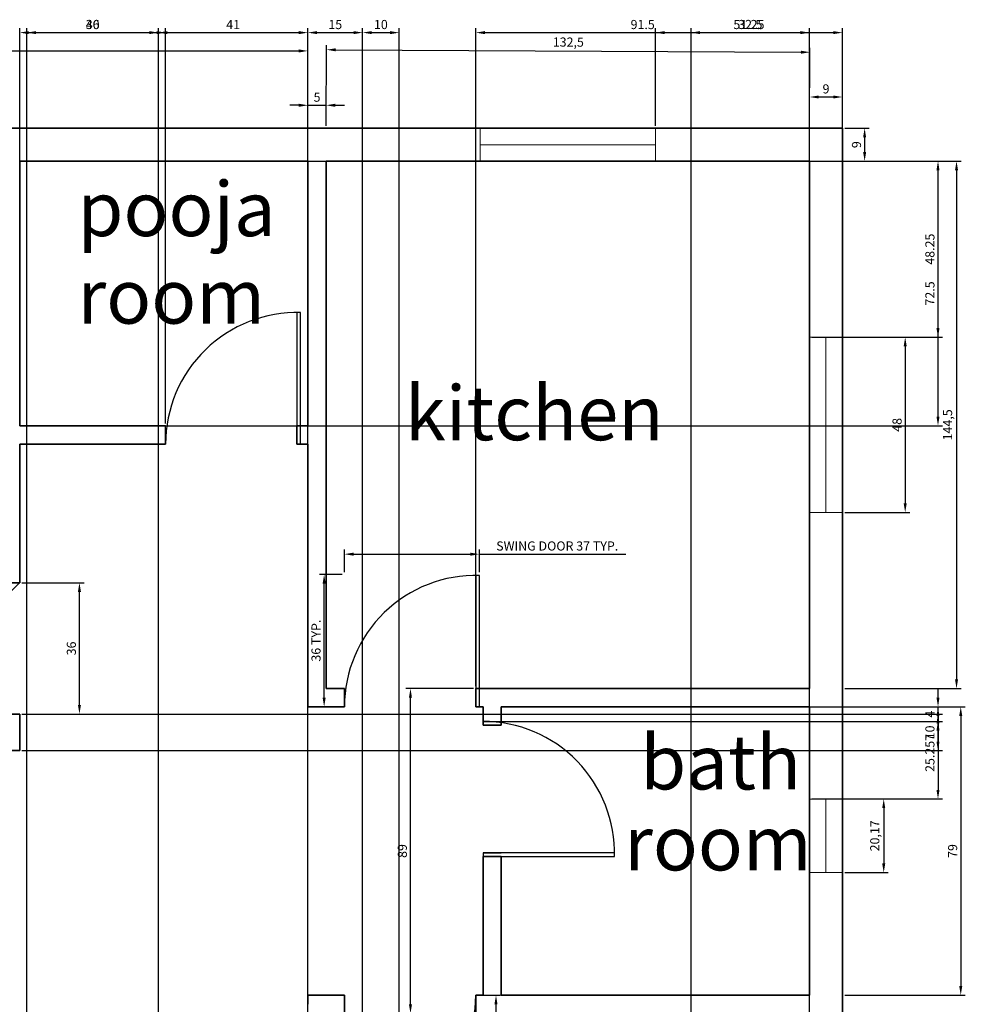
# Model space of a CAD drawing. Units: inches. Extents: x 64 to 791, y 453 to 990.
# Tile 3 of 3: x 531 to 791, y 721 to 990. Entities that reach past the tile are written whole.
import ezdxf

# ---------------------------------------------------------------- set-up
doc = ezdxf.new("R2010")
doc.units = ezdxf.units.IN
for name, color, linetype, lineweight in [('A-ANNO-DIMS', 2, 'Continuous', 18), ('A-AREA-IDEN', 7, 'Continuous', 25), ('A-DOOR', 3, 'Continuous', 25), ('A-GLAZ', 4, 'Continuous', 18), ('A-WALL', 7, 'Continuous', 35)]:
    doc.layers.add(name, color=color, linetype=linetype, lineweight=lineweight)
doc.styles.get("Standard").update_dxf_attribs({"font": 'arial.ttf'})
doc.dimstyles.new('ISO-25', dxfattribs={"dimtxt": 2.5, "dimasz": 2.5, "dimexe": 1.25, "dimexo": 0.625, "dimtad": 1, "dimtxsty": 'Standard', "dimcen": 2.5, "dimadec": 0, "dimazin": 0, "dimtfac": 1, "dimtmove": 0, "dimatfit": 3, "dimfxl": 1, "dimarcsym": 0})

# ---------------------------------------------------------------- blocks, each defined once
blk = doc.blocks.new('*D1')
at = {"layer": 'A-ANNO-DIMS', "color": 0, "lineweight": -2, "transparency": 16777216}
for p, q in [((757.56, 903.43), (775.4, 903.43)), ((774.15, 900.93), (774.15, 857.93)), ((757.56, 855.43), (775.4, 855.43))]:
    blk.add_line(p, q, dxfattribs=at)
at = {"layer": 'A-ANNO-DIMS', "color": 0, "transparency": 16777216}
for points in [[(773.73, 900.93), (774.56, 900.93), (774.15, 903.43)], [(773.73, 857.93), (774.56, 857.93), (774.15, 855.43)]]:
    blk.add_solid(points, dxfattribs=at)
at = {"layer": 'Defpoints', "color": 0, "transparency": 16777216}
for p in [(756.94, 903.43), (756.94, 855.43), (774.15, 855.43)]:
    blk.add_point(p, dxfattribs=at)
at = {"layer": 'A-ANNO-DIMS', "color": 0, "transparency": 16777216, "insert": (772.24, 879.43), "char_height": 2.5, "attachment_point": 5, "rotation": 90}
blk.add_mtext('48', dxfattribs=at)
blk = doc.blocks.new('*D2')
at = {"layer": 'A-ANNO-DIMS', "color": 0, "lineweight": -2, "transparency": 16777216}
for p, q in [((757.56, 951.68), (789.46, 951.68)), ((788.21, 949.18), (788.21, 809.68)), ((757.56, 807.18), (789.46, 807.18))]:
    blk.add_line(p, q, dxfattribs=at)
at = {"layer": 'A-ANNO-DIMS', "color": 0, "transparency": 16777216}
for points in [[(787.8, 949.18), (788.63, 949.18), (788.21, 951.68)], [(787.8, 809.68), (788.63, 809.68), (788.21, 807.18)]]:
    blk.add_solid(points, dxfattribs=at)
at = {"layer": 'Defpoints', "color": 0, "transparency": 16777216}
for p in [(756.94, 951.68), (756.94, 807.18), (788.21, 807.18)]:
    blk.add_point(p, dxfattribs=at)
at = {"layer": 'A-ANNO-DIMS', "color": 0, "transparency": 16777216, "insert": (786.09, 879.43), "char_height": 2.5, "attachment_point": 5, "rotation": 90}
blk.add_mtext('144,5', dxfattribs=at)
blk = doc.blocks.new('*D3')
at = {"layer": 'A-ANNO-DIMS', "color": 0, "lineweight": -2, "transparency": 16777216}
for p, q in [((757.56, 960.68), (764.28, 960.68)), ((763.03, 958.18), (763.03, 954.18)), ((757.56, 951.68), (764.28, 951.68))]:
    blk.add_line(p, q, dxfattribs=at)
at = {"layer": 'A-ANNO-DIMS', "color": 0, "transparency": 16777216}
for points in [[(762.61, 958.18), (763.44, 958.18), (763.03, 960.68)], [(762.61, 954.18), (763.44, 954.18), (763.03, 951.68)]]:
    blk.add_solid(points, dxfattribs=at)
at = {"layer": 'Defpoints', "color": 0, "transparency": 16777216}
for p in [(756.94, 960.68), (756.94, 951.68), (763.03, 951.68)]:
    blk.add_point(p, dxfattribs=at)
at = {"layer": 'A-ANNO-DIMS', "color": 0, "transparency": 16777216, "insert": (761.12, 956.18), "char_height": 2.5, "attachment_point": 5, "rotation": 90}
blk.add_mtext('9', dxfattribs=at)
blk = doc.blocks.new('*D4')
at = {"layer": 'A-ANNO-DIMS', "color": 0, "lineweight": -2, "transparency": 16777216}
for p, q in [((747.94, 960.63), (747.94, 970.5)), ((750.44, 969.25), (754.44, 969.25)), ((756.94, 960.63), (756.94, 970.5))]:
    blk.add_line(p, q, dxfattribs=at)
at = {"layer": 'A-ANNO-DIMS', "color": 0, "transparency": 16777216}
for points in [[(750.44, 969.66), (750.44, 968.83), (747.94, 969.25)], [(754.44, 969.66), (754.44, 968.83), (756.94, 969.25)]]:
    blk.add_solid(points, dxfattribs=at)
at = {"layer": 'Defpoints', "color": 0, "transparency": 16777216}
for p in [(756.94, 969.25), (747.94, 960), (756.94, 960)]:
    blk.add_point(p, dxfattribs=at)
at = {"layer": 'A-ANNO-DIMS', "color": 0, "transparency": 16777216, "insert": (752.44, 971.15), "char_height": 2.5, "attachment_point": 5}
blk.add_mtext('9', dxfattribs=at)
blk = doc.blocks.new('*D5')
at = {"layer": 'A-ANNO-DIMS', "color": 0, "lineweight": -2, "transparency": 16777216}
for p, q in [((615.44, 961.31), (615.55, 983.44)), ((618.05, 982.18), (745.55, 981.52)), ((747.94, 960.63), (748.05, 982.76))]:
    blk.add_line(p, q, dxfattribs=at)
at = {"layer": 'A-ANNO-DIMS', "color": 0, "transparency": 16777216}
for points in [[(618.05, 982.59), (618.05, 981.76), (615.55, 982.19)], [(745.55, 981.94), (745.55, 981.1), (748.05, 981.51)]]:
    blk.add_solid(points, dxfattribs=at)
at = {"layer": 'Defpoints', "color": 0, "transparency": 16777216}
for p in [(748.05, 981.51), (615.44, 960.68), (747.94, 960)]:
    blk.add_point(p, dxfattribs=at)
at = {"layer": 'A-ANNO-DIMS', "color": 0, "transparency": 16777216, "insert": (681.81, 983.97), "char_height": 2.5, "attachment_point": 5, "rotation": 359.7046}
blk.add_mtext('132,5', dxfattribs=at)
blk = doc.blocks.new('*D6')
at = {"layer": 'A-ANNO-DIMS', "color": 0, "lineweight": -2, "transparency": 16777216}
for p, q in [((607.94, 966.98), (605.44, 966.98)), ((610.44, 961.31), (610.44, 968.23)), ((610.44, 966.98), (615.44, 966.98)), ((615.44, 961.31), (615.44, 968.23)), ((617.94, 966.98), (620.44, 966.98))]:
    blk.add_line(p, q, dxfattribs=at)
at = {"layer": 'A-ANNO-DIMS', "color": 0, "transparency": 16777216}
for points in [[(607.94, 967.4), (607.94, 966.56), (610.44, 966.98)], [(617.94, 967.4), (617.94, 966.56), (615.44, 966.98)]]:
    blk.add_solid(points, dxfattribs=at)
at = {"layer": 'Defpoints', "color": 0, "transparency": 16777216}
for p in [(615.44, 966.98), (610.44, 960.68), (615.44, 960.68)]:
    blk.add_point(p, dxfattribs=at)
at = {"layer": 'A-ANNO-DIMS', "color": 0, "transparency": 16777216, "insert": (612.94, 968.88), "char_height": 2.5, "attachment_point": 5}
blk.add_mtext('5', dxfattribs=at)
blk = doc.blocks.new('*D7')
at = {"layer": 'A-ANNO-DIMS', "color": 0, "lineweight": -2, "transparency": 16777216}
for p, q in [((405.94, 961.31), (405.94, 983.12)), ((408.44, 981.87), (607.94, 981.87)), ((610.44, 961.31), (610.44, 983.12))]:
    blk.add_line(p, q, dxfattribs=at)
at = {"layer": 'A-ANNO-DIMS', "color": 0, "transparency": 16777216}
for points in [[(408.44, 982.28), (408.44, 981.45), (405.94, 981.87)], [(607.94, 982.28), (607.94, 981.45), (610.44, 981.87)]]:
    blk.add_solid(points, dxfattribs=at)
at = {"layer": 'Defpoints', "color": 0, "transparency": 16777216}
for p in [(610.44, 981.87), (405.94, 960.68), (610.44, 960.68)]:
    blk.add_point(p, dxfattribs=at)
at = {"layer": 'A-ANNO-DIMS', "color": 0, "transparency": 16777216, "insert": (508.19, 984), "char_height": 2.5, "attachment_point": 5}
blk.add_mtext('204,5', dxfattribs=at)
blk = doc.blocks.new('*D11')
at = {"layer": 'A-ANNO-DIMS', "color": 0, "lineweight": -2, "transparency": 16777216}
for p, q in [((757.56, 802.18), (790.62, 802.18)), ((789.37, 799.68), (789.37, 725.68)), ((757.56, 723.18), (790.62, 723.18))]:
    blk.add_line(p, q, dxfattribs=at)
at = {"layer": 'A-ANNO-DIMS', "color": 0, "transparency": 16777216}
for points in [[(788.96, 799.68), (789.79, 799.68), (789.37, 802.18)], [(788.96, 725.68), (789.79, 725.68), (789.37, 723.18)]]:
    blk.add_solid(points, dxfattribs=at)
at = {"layer": 'Defpoints', "color": 0, "transparency": 16777216}
for p in [(756.94, 802.18), (756.94, 723.18), (789.37, 723.18)]:
    blk.add_point(p, dxfattribs=at)
at = {"layer": 'A-ANNO-DIMS', "color": 0, "transparency": 16777216, "insert": (787.47, 762.68), "char_height": 2.5, "attachment_point": 5, "rotation": 90}
blk.add_mtext('79', dxfattribs=at)
blk = doc.blocks.new('*D12')
at = {"layer": 'A-ANNO-DIMS', "color": 0, "lineweight": -2, "transparency": 16777216}
for p, q in [((757.56, 776.93), (769.51, 776.93)), ((768.26, 774.43), (768.26, 759.26)), ((757.56, 756.76), (769.51, 756.76))]:
    blk.add_line(p, q, dxfattribs=at)
at = {"layer": 'A-ANNO-DIMS', "color": 0, "transparency": 16777216}
for points in [[(767.84, 774.43), (768.68, 774.43), (768.26, 776.93)], [(767.84, 759.26), (768.68, 759.26), (768.26, 756.76)]]:
    blk.add_solid(points, dxfattribs=at)
at = {"layer": 'Defpoints', "color": 0, "transparency": 16777216}
for p in [(756.94, 776.93), (756.94, 756.76), (768.26, 756.76)]:
    blk.add_point(p, dxfattribs=at)
at = {"layer": 'A-ANNO-DIMS', "color": 0, "transparency": 16777216, "insert": (766.13, 766.84), "char_height": 2.5, "attachment_point": 5, "rotation": 90}
blk.add_mtext('20,17', dxfattribs=at)
blk = doc.blocks.new('*D13')
at = {"layer": 'A-ANNO-DIMS', "color": 0, "lineweight": -2, "transparency": 16777216}
for p, q in [((532.06, 836.18), (549.07, 836.18)), ((547.82, 802.68), (547.82, 833.68)), ((532.06, 800.18), (549.07, 800.18))]:
    blk.add_line(p, q, dxfattribs=at)
at = {"layer": 'A-ANNO-DIMS', "color": 0, "transparency": 16777216}
for points in [[(547.4, 833.68), (548.23, 833.68), (547.82, 836.18)], [(547.4, 802.68), (548.23, 802.68), (547.82, 800.18)]]:
    blk.add_solid(points, dxfattribs=at)
at = {"layer": 'Defpoints', "color": 0, "transparency": 16777216}
for p in [(531.44, 836.18), (547.82, 836.18), (531.44, 800.18)]:
    blk.add_point(p, dxfattribs=at)
at = {"layer": 'A-ANNO-DIMS', "color": 0, "transparency": 16777216, "insert": (545.92, 818.18), "char_height": 2.5, "attachment_point": 5, "rotation": 90}
blk.add_mtext('36', dxfattribs=at)
blk = doc.blocks.new('*D23')
at = {"layer": 'A-ANNO-DIMS', "color": 0, "lineweight": -2, "transparency": 16777216}
for p, q in [((655.81, 807.18), (637.3, 807.18)), ((638.55, 720.68), (638.55, 804.68)), ((655.81, 718.18), (637.3, 718.18))]:
    blk.add_line(p, q, dxfattribs=at)
at = {"layer": 'A-ANNO-DIMS', "color": 0, "transparency": 16777216}
for points in [[(638.13, 804.68), (638.96, 804.68), (638.55, 807.18)], [(638.13, 720.68), (638.96, 720.68), (638.55, 718.18)]]:
    blk.add_solid(points, dxfattribs=at)
at = {"layer": 'Defpoints', "color": 0, "transparency": 16777216}
for p in [(638.55, 807.18), (656.44, 807.18), (656.44, 718.18)]:
    blk.add_point(p, dxfattribs=at)
at = {"layer": 'A-ANNO-DIMS', "color": 0, "transparency": 16777216, "insert": (636.64, 762.68), "char_height": 2.5, "attachment_point": 5, "rotation": 90}
blk.add_mtext('89', dxfattribs=at)
blk = doc.blocks.new('WIN-48IN')
for p, q in [((0, 48), (9, 48)), ((4.5, 48), (4.5, 0)), ((0, 0), (9, 0))]:
    blk.add_line(p, q)
blk = doc.blocks.new('DOOR-SWING-36IN')
for p, q in [((0, 0), (0, 5)), ((36, 0), (36, 5))]:
    blk.add_line(p, q)
blk.add_lwpolyline([(36, 0), (37, 0), (37, 36), (36, 36)], close=True)
blk.add_arc((36.01, 0), 36.01, 88.4304, 180)
blk = doc.blocks.new('DOOR-SWING-36IN-OPEN-PROFILE')
for p, q in [((0, 0), (0, 5)), ((36, 0), (36, 5))]:
    blk.add_line(p, q)
blk.add_lwpolyline([(37, 5), (37, 36), (36, 36), (36, 0), (37, 0)])
blk.add_arc((36.01, 0), 36.01, 88.4304, 180)
blk = doc.blocks.new('*D28')
at = {"layer": 'A-ANNO-DIMS', "color": 0, "lineweight": -2, "transparency": 16777216}
for p, q in [((620.44, 839.07), (620.44, 845.25)), ((657.44, 839.07), (657.44, 845.25)), ((622.94, 844), (654.94, 844)), ((657.44, 844), (697.6, 844))]:
    blk.add_line(p, q, dxfattribs=at)
at = {"layer": 'A-ANNO-DIMS', "color": 0, "transparency": 16777216}
for points in [[(622.94, 844.42), (622.94, 843.58), (620.44, 844)], [(654.94, 844.42), (654.94, 843.58), (657.44, 844)]]:
    blk.add_solid(points, dxfattribs=at)
at = {"layer": 'Defpoints', "color": 0, "transparency": 16777216}
for p in [(657.44, 844), (620.44, 838.45), (657.44, 838.45)]:
    blk.add_point(p, dxfattribs=at)
at = {"layer": 'A-ANNO-DIMS', "color": 0, "transparency": 16777216, "insert": (678.77, 845.92), "char_height": 2.5, "attachment_point": 5}
blk.add_mtext('SWING DOOR 37 TYP.', dxfattribs=at)
blk = doc.blocks.new('*D29')
at = {"layer": 'A-ANNO-DIMS', "color": 0, "lineweight": -2, "transparency": 16777216}
for p, q in [((619.81, 838.45), (613.64, 838.45)), ((614.89, 804.68), (614.89, 835.95)), ((619.81, 802.18), (613.64, 802.18))]:
    blk.add_line(p, q, dxfattribs=at)
at = {"layer": 'A-ANNO-DIMS', "color": 0, "transparency": 16777216}
for points in [[(614.47, 835.95), (615.3, 835.95), (614.89, 838.45)], [(614.47, 804.68), (615.3, 804.68), (614.89, 802.18)]]:
    blk.add_solid(points, dxfattribs=at)
at = {"layer": 'Defpoints', "color": 0, "transparency": 16777216}
for p in [(614.89, 838.45), (620.44, 838.45), (620.44, 802.18)]:
    blk.add_point(p, dxfattribs=at)
at = {"layer": 'A-ANNO-DIMS', "color": 0, "transparency": 16777216, "insert": (612.98, 820.32), "char_height": 2.5, "attachment_point": 5, "rotation": 90}
blk.add_mtext('36 TYP.', dxfattribs=at)
blk = doc.blocks.new('*D31')
at = {"layer": 'A-ANNO-DIMS', "color": 0, "lineweight": -2, "transparency": 16777216}
for p, q in [((657.06, 723.18), (663.24, 723.18)), ((661.99, 720.68), (661.99, 689.42)), ((657.06, 686.92), (663.24, 686.92))]:
    blk.add_line(p, q, dxfattribs=at)
at = {"layer": 'A-ANNO-DIMS', "color": 0, "transparency": 16777216}
for points in [[(661.57, 720.68), (662.4, 720.68), (661.99, 723.18)], [(661.57, 689.42), (662.4, 689.42), (661.99, 686.92)]]:
    blk.add_solid(points, dxfattribs=at)
at = {"layer": 'Defpoints', "color": 0, "transparency": 16777216}
for p in [(656.44, 723.18), (656.44, 686.92), (661.99, 686.92)]:
    blk.add_point(p, dxfattribs=at)
at = {"layer": 'A-ANNO-DIMS', "color": 0, "transparency": 16777216, "insert": (660.08, 705.05), "char_height": 2.5, "attachment_point": 5, "rotation": 90}
blk.add_mtext('36 TYP.', dxfattribs=at)
blk = doc.blocks.new('*D35')
at = {"layer": 'A-ANNO-DIMS', "color": 0, "lineweight": -2, "transparency": 16777216}
for p, q in [((532.06, 951.68), (784.39, 951.68)), ((783.14, 881.68), (783.14, 949.18)), ((532.06, 879.18), (784.39, 879.18))]:
    blk.add_line(p, q, dxfattribs=at)
at = {"layer": 'A-ANNO-DIMS', "color": 0, "transparency": 16777216}
for points in [[(782.72, 949.18), (783.55, 949.18), (783.14, 951.68)], [(782.72, 881.68), (783.55, 881.68), (783.14, 879.18)]]:
    blk.add_solid(points, dxfattribs=at)
at = {"layer": 'Defpoints', "color": 0, "transparency": 16777216}
for p in [(531.44, 951.68), (783.14, 951.68), (531.44, 879.18)]:
    blk.add_point(p, dxfattribs=at)
at = {"layer": 'A-ANNO-DIMS', "color": 0, "transparency": 16777216, "insert": (781.24, 915.43), "char_height": 2.5, "attachment_point": 5, "rotation": 90}
blk.add_mtext('72.5', dxfattribs=at)
blk = doc.blocks.new('*D38')
at = {"layer": 'A-ANNO-DIMS', "color": 0, "lineweight": -2, "transparency": 16777216}
for p, q in [((705.69, 961.31), (705.69, 988.13)), ((756.94, 961.31), (756.94, 988.13)), ((708.19, 986.88), (754.44, 986.88))]:
    blk.add_line(p, q, dxfattribs=at)
at = {"layer": 'A-ANNO-DIMS', "color": 0, "transparency": 16777216}
for points in [[(708.19, 987.3), (708.19, 986.47), (705.69, 986.88)], [(754.44, 987.3), (754.44, 986.47), (756.94, 986.88)]]:
    blk.add_solid(points, dxfattribs=at)
at = {"layer": 'Defpoints', "color": 0, "transparency": 16777216}
for p in [(756.94, 986.88), (705.69, 960.68), (756.94, 960.68)]:
    blk.add_point(p, dxfattribs=at)
at = {"layer": 'A-ANNO-DIMS', "color": 0, "transparency": 16777216, "insert": (731.31, 988.78), "char_height": 2.5, "attachment_point": 5}
blk.add_mtext('51.25', dxfattribs=at)
blk = doc.blocks.new('*D41')
at = {"layer": 'A-ANNO-DIMS', "color": 0, "lineweight": -2, "transparency": 16777216}
for p, q in [((748.56, 802.18), (784.39, 802.18)), ((783.14, 799.68), (783.14, 779.43)), ((748.56, 776.93), (784.39, 776.93))]:
    blk.add_line(p, q, dxfattribs=at)
at = {"layer": 'A-ANNO-DIMS', "color": 0, "transparency": 16777216}
for points in [[(782.72, 799.68), (783.55, 799.68), (783.14, 802.18)], [(782.72, 779.43), (783.55, 779.43), (783.14, 776.93)]]:
    blk.add_solid(points, dxfattribs=at)
at = {"layer": 'Defpoints', "color": 0, "transparency": 16777216}
for p in [(747.94, 802.18), (747.94, 776.93), (783.14, 776.93)]:
    blk.add_point(p, dxfattribs=at)
at = {"layer": 'A-ANNO-DIMS', "color": 0, "transparency": 16777216, "insert": (781.24, 789.55), "char_height": 2.5, "attachment_point": 5, "rotation": 90}
blk.add_mtext('25.257', dxfattribs=at)
blk = doc.blocks.new('*D42')
at = {"layer": 'A-ANNO-DIMS', "color": 0, "lineweight": -2, "transparency": 16777216}
for p, q in [((748.56, 951.68), (784.39, 951.68)), ((783.14, 905.93), (783.14, 949.18)), ((748.56, 903.43), (784.39, 903.43))]:
    blk.add_line(p, q, dxfattribs=at)
at = {"layer": 'A-ANNO-DIMS', "color": 0, "transparency": 16777216}
for points in [[(782.72, 949.18), (783.55, 949.18), (783.14, 951.68)], [(782.72, 905.93), (783.55, 905.93), (783.14, 903.43)]]:
    blk.add_solid(points, dxfattribs=at)
at = {"layer": 'Defpoints', "color": 0, "transparency": 16777216}
for p in [(747.94, 951.68), (783.14, 951.68), (747.94, 903.43)]:
    blk.add_point(p, dxfattribs=at)
at = {"layer": 'A-ANNO-DIMS', "color": 0, "transparency": 16777216, "insert": (781.24, 927.56), "char_height": 2.5, "attachment_point": 5, "rotation": 90}
blk.add_mtext('48.25', dxfattribs=at)
blk = doc.blocks.new('*D43')
at = {"layer": 'A-ANNO-DIMS', "color": 0, "lineweight": -2, "transparency": 16777216}
for p, q in [((569.44, 562.81), (569.44, 988.13)), ((610.44, 567.81), (610.44, 988.13)), ((571.94, 986.88), (607.94, 986.88))]:
    blk.add_line(p, q, dxfattribs=at)
at = {"layer": 'A-ANNO-DIMS', "color": 0, "transparency": 16777216}
for points in [[(571.94, 987.3), (571.94, 986.47), (569.44, 986.88)], [(607.94, 987.3), (607.94, 986.47), (610.44, 986.88)]]:
    blk.add_solid(points, dxfattribs=at)
at = {"layer": 'Defpoints', "color": 0, "transparency": 16777216}
for p in [(610.44, 986.88), (610.44, 567.18), (569.44, 562.18)]:
    blk.add_point(p, dxfattribs=at)
at = {"layer": 'A-ANNO-DIMS', "color": 0, "transparency": 16777216, "insert": (589.94, 988.76), "char_height": 2.5, "attachment_point": 5}
blk.add_mtext('41', dxfattribs=at)
blk = doc.blocks.new('*D44')
at = {"layer": 'A-ANNO-DIMS', "color": 0, "lineweight": -2, "transparency": 16777216}
for p, q in [((533.44, 567.81), (533.44, 988.13)), ((569.44, 562.81), (569.44, 988.13)), ((535.94, 986.88), (566.94, 986.88))]:
    blk.add_line(p, q, dxfattribs=at)
at = {"layer": 'A-ANNO-DIMS', "color": 0, "transparency": 16777216}
for points in [[(535.94, 987.3), (535.94, 986.47), (533.44, 986.88)], [(566.94, 987.3), (566.94, 986.47), (569.44, 986.88)]]:
    blk.add_solid(points, dxfattribs=at)
at = {"layer": 'Defpoints', "color": 0, "transparency": 16777216}
for p in [(569.44, 986.88), (533.44, 567.18), (569.44, 562.18)]:
    blk.add_point(p, dxfattribs=at)
at = {"layer": 'A-ANNO-DIMS', "color": 0, "transparency": 16777216, "insert": (551.44, 988.79), "char_height": 2.5, "attachment_point": 5}
blk.add_mtext('36', dxfattribs=at)
blk = doc.blocks.new('*D45')
at = {"layer": 'A-ANNO-DIMS', "color": 0, "lineweight": -2, "transparency": 16777216}
for p, q in [((625.44, 490.31), (625.44, 988.13)), ((635.44, 490.31), (635.44, 988.13)), ((627.94, 986.88), (632.94, 986.88))]:
    blk.add_line(p, q, dxfattribs=at)
at = {"layer": 'A-ANNO-DIMS', "color": 0, "transparency": 16777216}
for points in [[(627.94, 987.3), (627.94, 986.47), (625.44, 986.88)], [(632.94, 987.3), (632.94, 986.47), (635.44, 986.88)]]:
    blk.add_solid(points, dxfattribs=at)
at = {"layer": 'Defpoints', "color": 0, "transparency": 16777216}
for p in [(635.44, 986.88), (625.44, 489.68), (635.44, 489.68)]:
    blk.add_point(p, dxfattribs=at)
at = {"layer": 'A-ANNO-DIMS', "color": 0, "transparency": 16777216, "insert": (630.44, 988.78), "char_height": 2.5, "attachment_point": 5}
blk.add_mtext('10', dxfattribs=at)
blk = doc.blocks.new('*D46')
at = {"layer": 'A-ANNO-DIMS', "color": 0, "lineweight": -2, "transparency": 16777216}
for p, q in [((610.44, 490.31), (610.44, 988.13)), ((625.44, 490.31), (625.44, 988.13)), ((612.94, 986.88), (622.94, 986.88))]:
    blk.add_line(p, q, dxfattribs=at)
at = {"layer": 'A-ANNO-DIMS', "color": 0, "transparency": 16777216}
for points in [[(612.94, 987.3), (612.94, 986.47), (610.44, 986.88)], [(622.94, 987.3), (622.94, 986.47), (625.44, 986.88)]]:
    blk.add_solid(points, dxfattribs=at)
at = {"layer": 'Defpoints', "color": 0, "transparency": 16777216}
for p in [(625.44, 986.88), (610.44, 489.68), (625.44, 489.68)]:
    blk.add_point(p, dxfattribs=at)
at = {"layer": 'A-ANNO-DIMS', "color": 0, "transparency": 16777216, "insert": (617.94, 988.78), "char_height": 2.5, "attachment_point": 5}
blk.add_mtext('15', dxfattribs=at)
blk = doc.blocks.new('*D47')
at = {"layer": 'A-ANNO-DIMS', "color": 0, "lineweight": -2, "transparency": 16777216}
for p, q in [((715.44, 490.31), (715.44, 988.13)), ((747.94, 490.31), (747.94, 988.13)), ((717.94, 986.88), (745.44, 986.88))]:
    blk.add_line(p, q, dxfattribs=at)
at = {"layer": 'A-ANNO-DIMS', "color": 0, "transparency": 16777216}
for points in [[(717.94, 987.3), (717.94, 986.47), (715.44, 986.88)], [(745.44, 987.3), (745.44, 986.47), (747.94, 986.88)]]:
    blk.add_solid(points, dxfattribs=at)
at = {"layer": 'Defpoints', "color": 0, "transparency": 16777216}
for p in [(747.94, 986.88), (715.44, 489.68), (747.94, 489.68)]:
    blk.add_point(p, dxfattribs=at)
at = {"layer": 'A-ANNO-DIMS', "color": 0, "transparency": 16777216, "insert": (731.69, 988.79), "char_height": 2.5, "attachment_point": 5}
blk.add_mtext('32.5', dxfattribs=at)
blk = doc.blocks.new('*D49')
at = {"layer": 'A-ANNO-DIMS', "color": 0, "lineweight": -2, "transparency": 16777216}
for p, q in [((531.44, 879.81), (531.44, 988.13)), ((571.44, 879.81), (571.44, 988.13)), ((533.94, 986.88), (568.94, 986.88))]:
    blk.add_line(p, q, dxfattribs=at)
at = {"layer": 'A-ANNO-DIMS', "color": 0, "transparency": 16777216}
for points in [[(533.94, 987.3), (533.94, 986.47), (531.44, 986.88)], [(568.94, 987.3), (568.94, 986.47), (571.44, 986.88)]]:
    blk.add_solid(points, dxfattribs=at)
at = {"layer": 'Defpoints', "color": 0, "transparency": 16777216}
for p in [(571.44, 986.88), (531.44, 879.18), (571.44, 879.18)]:
    blk.add_point(p, dxfattribs=at)
at = {"layer": 'A-ANNO-DIMS', "color": 0, "transparency": 16777216, "insert": (551.44, 988.78), "char_height": 2.5, "attachment_point": 5}
blk.add_mtext('40', dxfattribs=at)
blk = doc.blocks.new('*D50')
at = {"layer": 'A-ANNO-DIMS', "color": 0, "lineweight": -2, "transparency": 16777216}
for p, q in [((656.44, 807.81), (656.44, 988.13)), ((747.94, 807.81), (747.94, 988.13)), ((658.94, 986.88), (745.44, 986.88))]:
    blk.add_line(p, q, dxfattribs=at)
at = {"layer": 'A-ANNO-DIMS', "color": 0, "transparency": 16777216}
for points in [[(658.94, 987.3), (658.94, 986.47), (656.44, 986.88)], [(745.44, 987.3), (745.44, 986.47), (747.94, 986.88)]]:
    blk.add_solid(points, dxfattribs=at)
at = {"layer": 'Defpoints', "color": 0, "transparency": 16777216}
for p in [(747.94, 986.88), (656.44, 807.18), (747.94, 807.18)]:
    blk.add_point(p, dxfattribs=at)
at = {"layer": 'A-ANNO-DIMS', "color": 0, "transparency": 16777216, "insert": (702.19, 988.78), "char_height": 2.5, "attachment_point": 5}
blk.add_mtext('91.5', dxfattribs=at)
blk = doc.blocks.new('*D51')
at = {"layer": 'A-ANNO-DIMS', "color": 0, "lineweight": -2, "transparency": 16777216}
for p, q in [((783.14, 804.68), (783.14, 807.18)), ((664.06, 802.18), (784.39, 802.18)), ((783.14, 798.18), (783.14, 802.18)), ((659.06, 798.18), (784.39, 798.18)), ((783.14, 795.68), (783.14, 793.18))]:
    blk.add_line(p, q, dxfattribs=at)
at = {"layer": 'A-ANNO-DIMS', "color": 0, "transparency": 16777216}
for points in [[(782.72, 804.68), (783.55, 804.68), (783.14, 802.18)], [(782.72, 795.68), (783.55, 795.68), (783.14, 798.18)]]:
    blk.add_solid(points, dxfattribs=at)
at = {"layer": 'Defpoints', "color": 0, "transparency": 16777216}
for p in [(663.44, 802.18), (783.14, 802.18), (658.44, 798.18)]:
    blk.add_point(p, dxfattribs=at)
at = {"layer": 'A-ANNO-DIMS', "color": 0, "transparency": 16777216, "insert": (781.26, 800.18), "char_height": 2.5, "attachment_point": 5, "rotation": 90}
blk.add_mtext('4', dxfattribs=at)
blk = doc.blocks.new('*D52')
at = {"layer": 'A-ANNO-DIMS', "color": 0, "lineweight": -2, "transparency": 16777216}
for p, q in [((532.06, 800.18), (784.39, 800.18)), ((783.14, 792.68), (783.14, 797.68)), ((532.06, 790.18), (784.39, 790.18))]:
    blk.add_line(p, q, dxfattribs=at)
at = {"layer": 'A-ANNO-DIMS', "color": 0, "transparency": 16777216}
for points in [[(782.72, 797.68), (783.55, 797.68), (783.14, 800.18)], [(782.72, 792.68), (783.55, 792.68), (783.14, 790.18)]]:
    blk.add_solid(points, dxfattribs=at)
at = {"layer": 'Defpoints', "color": 0, "transparency": 16777216}
for p in [(531.44, 800.18), (783.14, 800.18), (531.44, 790.18)]:
    blk.add_point(p, dxfattribs=at)
at = {"layer": 'A-ANNO-DIMS', "color": 0, "transparency": 16777216, "insert": (781.24, 795.18), "char_height": 2.5, "attachment_point": 5, "rotation": 90}
blk.add_mtext('10', dxfattribs=at)
blk = doc.blocks.new('*D55')
at = {"layer": 'A-ANNO-DIMS', "color": 0, "lineweight": -2, "transparency": 16777216}
for p, q in [((531.44, 836.2), (505.62, 811.08)), ((484.05, 790.09), (503.83, 809.34))]:
    blk.add_line(p, q, dxfattribs=at)
at = {"layer": 'A-ANNO-DIMS', "color": 0, "transparency": 16777216}
blk.add_solid([(503.54, 809.64), (504.12, 809.04), (505.62, 811.08)], dxfattribs=at)
at = {"layer": 'Defpoints', "color": 0, "transparency": 16777216}
for p in [(531.44, 836.2), (505.62, 811.08)]:
    blk.add_point(p, dxfattribs=at)
at = {"layer": 'A-ANNO-DIMS', "color": 0, "transparency": 16777216, "insert": (488.81, 797.38), "char_height": 2.5, "attachment_point": 5, "rotation": 44.2145}
blk.add_mtext('6X R36.01', dxfattribs=at)

msp = doc.modelspace()

# ---------------------------------------------------------------- linework, layer by layer
at = {"layer": 'A-GLAZ'}
for p, q in [((747.937, 776.9261), (756.937, 776.9261)), ((752.437, 776.9261), (752.437, 756.7571)), ((756.937, 756.7571), (747.937, 756.7571)), ((752.437, 756.7571), (756.937, 756.7571))]:
    msp.add_line(p, q, dxfattribs=at)
at = {"layer": 'A-WALL'}
for p, q in [((756.937, 960.6832), (396.937, 960.6832)), ((528.937, 960.6832), (612.937, 960.6832)), ((612.937, 960.6832), (756.937, 960.6832)), ((756.937, 480.6832), (756.937, 960.6832)), ((531.437, 951.6832), (531.437, 879.1832)), ((610.437, 951.6832), (531.437, 951.6832)), ((610.437, 879.1832), (610.437, 951.6832)), ((747.937, 951.6832), (615.437, 951.6832)), ((615.437, 807.1832), (615.437, 951.6832)), ((615.437, 951.6832), (747.937, 951.6832)), ((747.937, 951.6832), (632.5937, 951.6832)), ((747.937, 951.6832), (747.937, 807.1832)), ((747.937, 807.1832), (747.937, 951.6832)), ((571.437, 879.1832), (531.437, 879.1832)), ((607.437, 879.1832), (610.437, 879.1832)), ((607.437, 874.1832), (607.437, 879.1832)), ((531.437, 874.1832), (531.437, 836.1832)), ((571.437, 874.1832), (531.437, 874.1832)), ((607.437, 874.1832), (610.437, 874.1832)), ((610.437, 802.1832), (610.437, 874.1832)), ((526.437, 836.1832), (531.437, 836.1832)), ((615.437, 807.1832), (620.437, 807.1832)), ((620.437, 807.1832), (620.437, 802.1832)), ((656.437, 807.1832), (656.437, 802.1832)), ((656.437, 807.1832), (747.937, 807.1832)), ((756.937, 804.6832), (756.937, 720.6832)), ((610.437, 802.1832), (620.437, 802.1832)), ((656.437, 802.1832), (658.437, 802.1832)), ((658.437, 802.1832), (658.437, 797.1832)), ((663.437, 802.1832), (663.437, 797.1832)), ((663.437, 802.1832), (747.937, 802.1832)), ((747.937, 723.1832), (747.937, 802.1832)), ((747.937, 723.1832), (747.937, 802.1832)), ((526.437, 800.1832), (531.437, 800.1832)), ((531.437, 800.1832), (531.437, 790.1832)), ((658.437, 797.1832), (663.437, 797.1832)), ((405.937, 790.1832), (531.437, 790.1832)), ((658.437, 761.1832), (663.437, 761.1832)), ((658.437, 761.1832), (658.437, 723.1832)), ((663.437, 761.1832), (663.437, 723.1832)), ((612.937, 723.1832), (610.437, 723.1832)), ((610.437, 723.1832), (610.437, 720.6832)), ((612.937, 723.1832), (620.437, 723.1832)), ((620.437, 718.1832), (620.437, 723.1832)), ((656.437, 718.1832), (656.437, 723.1832)), ((656.437, 723.1832), (658.437, 723.1832)), ((663.437, 723.1832), (747.937, 723.1832))]:
    msp.add_line(p, q, dxfattribs=at)

# ---------------------------------------------------------------- block references
at = {"layer": 'A-DOOR'}
for p in [(571.437, 874.183), (620.437, 802.183)]:
    msp.add_blockref('DOOR-SWING-36IN', p, dxfattribs=at)
for name, p, rotation in [('DOOR-SWING-36IN', (658.4368, 798.1832), 270.0000000000001), ('DOOR-SWING-36IN-OPEN-PROFILE', (656.437, 723.1834), 180)]:
    msp.add_blockref(name, p, dxfattribs=dict(at, rotation=rotation))
at = {"layer": 'A-GLAZ', "rotation": 269.9999999999999}
msp.add_blockref('WIN-48IN', (657.6866, 960.6832), dxfattribs=at)
at = {"layer": 'A-GLAZ'}
msp.add_blockref('WIN-48IN', (747.937, 855.4328), dxfattribs=at)

# ---------------------------------------------------------------- texts
at = {"layer": 'A-AREA-IDEN'}
for s, p in [('pooja', (547.2621, 931.135)), ('room ', (547.2621, 907.1609)), ('kitchen', (636.9841, 875.2153)), ('bath', (701.5346, 779.5487)), ('room', (697.095, 757.367))]:
    msp.add_text(s, height=14.92404, dxfattribs=at).set_placement(p)

# ---------------------------------------------------------------- dimensions: what is measured, and where the dimension line sits
at = {"layer": 'A-ANNO-DIMS'}
for base, p1, p2, override, picture, middle in [((571.437, 986.8832), (531.437, 879.1832), (571.437, 879.1832), {"dimdec": 0, "dimlfac": 1, "dimrnd": 0, "dimzin": 0, "dimdsep": 46, "dimlunit": 2}, '*D49', (551.437, 988.7846)), ((569.437, 986.8832), (533.437, 567.1832), (569.437, 562.1832), {"dimdec": 0, "dimlfac": 1, "dimrnd": 0, "dimzin": 0, "dimdsep": 46, "dimlunit": 2}, '*D44', (551.437, 988.7855)), ((610.437, 986.8832), (569.437, 562.1832), (610.437, 567.1832), {"dimdec": 0, "dimlfac": 1, "dimrnd": 0, "dimzin": 0, "dimdsep": 46, "dimlunit": 2}, '*D43', (589.937, 988.7633)), ((625.437, 986.8832), (610.437, 489.6832), (625.437, 489.6832), {"dimdec": 0, "dimlfac": 1, "dimrnd": 0, "dimzin": 0, "dimdsep": 46, "dimlunit": 2}, '*D46', (617.937, 988.7846)), ((635.437, 986.8832), (625.437, 489.6832), (635.437, 489.6832), {"dimdec": 0, "dimlfac": 1, "dimrnd": 0, "dimzin": 0, "dimdsep": 46, "dimlunit": 2}, '*D45', (630.437, 988.7846)), ((747.937, 986.8832), (656.437, 807.1832), (747.937, 807.1832), {"dimdec": 1, "dimlfac": 1, "dimrnd": 0, "dimzin": 0, "dimdsep": 46, "dimlunit": 2}, '*D50', (702.187, 988.7846)), ((756.937, 986.8832), (705.687, 960.6832), (756.937, 960.6832), {"dimdec": 2, "dimlfac": 1, "dimrnd": 0, "dimzin": 0, "dimdsep": 46, "dimlunit": 2}, '*D38', (731.312, 988.7846)), ((747.937, 986.8832), (715.437, 489.6832), (747.937, 489.6832), {"dimdec": 1, "dimlfac": 1, "dimrnd": 0, "dimzin": 0, "dimdsep": 46, "dimlunit": 2}, '*D47', (731.687, 988.7855)), ((610.437, 981.8679), (405.937, 960.6832), (610.437, 960.6832), {"dimclrd": 0, "dimclre": 0, "dimclrt": 0}, '*D7', (508.187, 983.9953)), ((756.937, 969.2459), (747.937, 960.0001), (756.937, 960.0001), {"dimclrd": 0, "dimclre": 0, "dimclrt": 0}, '*D4', (752.437, 971.1473)), ((615.437, 966.9789), (610.437, 960.6832), (615.437, 960.6832), {"dimclrd": 0, "dimclre": 0, "dimclrt": 0}, '*D6', (612.937, 968.8752))]:
    dim = msp.add_linear_dim(base=base, p1=p1, p2=p2, dimstyle='ISO-25', override=override, dxfattribs=at)
    dim.commit()
    dim.dimension.update_dxf_attribs({"geometry": picture, "text_midpoint": middle})
dim = msp.add_aligned_dim(p1=(615.437, 960.6832), p2=(747.937, 960.0001), distance=21.5057, dimstyle='ISO-25', override={"dimclrd": 0, "dimclre": 0, "dimclrt": 0}, dxfattribs=at)
dim.commit()
dim.dimension.update_dxf_attribs({"geometry": '*D5', "text_midpoint": (681.8088, 983.9744)})
for base, p1, p2, override, picture, middle in [((763.0252, 951.6832), (756.937, 960.6832), (756.937, 951.6832), {"dimclrd": 0, "dimclre": 0, "dimclrt": 0}, '*D3', (761.1237, 956.1832)), ((783.137, 951.6832), (531.437, 879.1832), (531.437, 951.6832), {"dimdec": 1, "dimlfac": 1, "dimrnd": 0, "dimzin": 0, "dimdsep": 46, "dimlunit": 2}, '*D35', (781.2355, 915.4332)), ((783.137, 951.6832), (747.937, 903.4332), (747.937, 951.6832), {"dimdec": 2, "dimlfac": 1, "dimrnd": 0, "dimzin": 0, "dimdsep": 46, "dimlunit": 2}, '*D42', (781.2355, 927.5582)), ((788.2135, 807.1832), (756.937, 951.6832), (756.937, 807.1832), {"dimclrd": 0, "dimclre": 0, "dimclrt": 0}, '*D2', (786.0861, 879.4332)), ((774.146, 855.4332), (756.937, 903.4332), (756.937, 855.4332), {"dimclrd": 0, "dimclre": 0, "dimclrt": 0}, '*D1', (772.2446, 879.4332)), ((547.8176, 836.1832), (531.437, 800.1832), (531.437, 836.1832), {"dimclrd": 0, "dimclre": 0, "dimclrt": 0}, '*D13', (545.9153, 818.1832)), ((638.5461, 807.1832), (656.437, 718.1832), (656.437, 807.1832), {"dimclrd": 0, "dimclre": 0, "dimclrt": 0}, '*D23', (636.6447, 762.6832)), ((783.137, 802.1832), (658.437, 798.1832), (663.437, 802.1832), {"dimdec": 0, "dimlfac": 1, "dimrnd": 0, "dimzin": 0, "dimdsep": 46, "dimlunit": 2}, '*D51', (781.262, 800.1832)), ((783.137, 776.9261), (747.937, 802.1832), (747.937, 776.9261), {"dimdec": 3, "dimlfac": 1, "dimrnd": 0, "dimzin": 0, "dimdsep": 46, "dimlunit": 2}, '*D41', (781.2355, 789.5546)), ((789.3748, 723.1832), (756.937, 802.1832), (756.937, 723.1832), {"dimclrd": 0, "dimclre": 0, "dimclrt": 0}, '*D11', (787.4734, 762.6832)), ((783.137, 800.1832), (531.437, 790.1832), (531.437, 800.1832), {"dimdec": 0, "dimlfac": 1, "dimrnd": 0, "dimzin": 0, "dimdsep": 46, "dimlunit": 2}, '*D52', (781.2355, 795.1832)), ((768.2603, 756.7571), (756.937, 776.9261), (756.937, 756.7571), {"dimclrd": 0, "dimclre": 0, "dimclrt": 0}, '*D12', (766.1329, 766.8416))]:
    dim = msp.add_linear_dim(base=base, p1=p1, p2=p2, angle=90, dimstyle='ISO-25', override=override, dxfattribs=at)
    dim.commit()
    dim.dimension.update_dxf_attribs({"geometry": picture, "text_midpoint": middle})
dim = msp.add_linear_dim(base=(657.437, 843.9995), p1=(620.437, 838.4495), p2=(657.437, 838.4495), text='SWING DOOR <> TYP.', dimstyle='ISO-25', override={"dimdec": 0, "dimlfac": 1, "dimrnd": 0, "dimzin": 0, "dimdsep": 46, "dimlunit": 2}, dxfattribs=at)
dim.commit()
dim.dimension.update_dxf_attribs({"geometry": '*D28', "text_midpoint": (678.7671, 845.9189)})
for base, p1, p2, angle, picture, middle in [((614.887, 838.4495), (620.437, 802.1832), (620.437, 838.4495), 90, '*D29', (612.9847, 820.3164)), ((661.987, 686.9169), (656.437, 723.1832), (656.437, 686.9169), 270, '*D31', (660.0847, 705.0501))]:
    dim = msp.add_linear_dim(base=base, p1=p1, p2=p2, angle=angle, text='<> TYP.', dimstyle='ISO-25', override={"dimdec": 0, "dimlfac": 1, "dimrnd": 0, "dimzin": 0, "dimdsep": 46, "dimlunit": 2}, dxfattribs=at)
    dim.commit()
    dim.dimension.update_dxf_attribs({"geometry": picture, "text_midpoint": middle})
dim = msp.add_radius_dim(center=(531.437, 836.1967), mpoint=(505.6248, 811.0828), text='6X <>', dimstyle='ISO-25', override={"dimdec": 2, "dimlfac": 1, "dimrnd": 0, "dimzin": 0, "dimdsep": 46, "dimlunit": 2}, dxfattribs=at)
dim.commit()
dim.dimension.update_dxf_attribs({"geometry": '*D55', "text_midpoint": (490.1376, 796.0145), "dimtype": 164})

doc.saveas('drawing.dxf')
